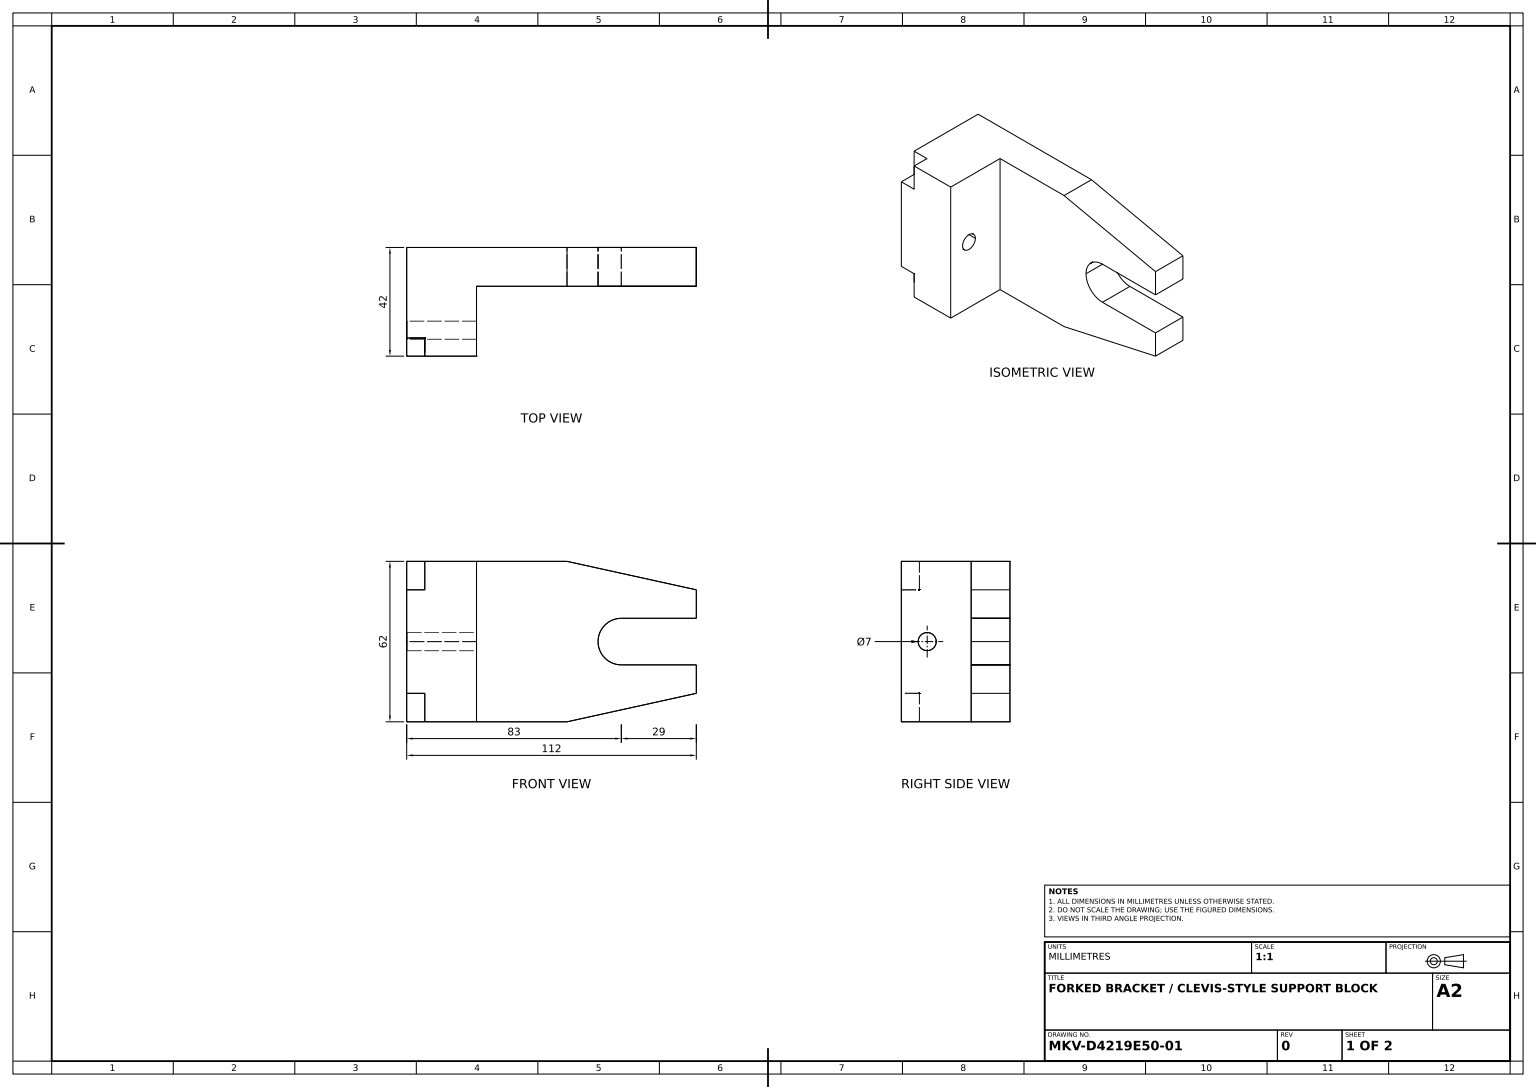
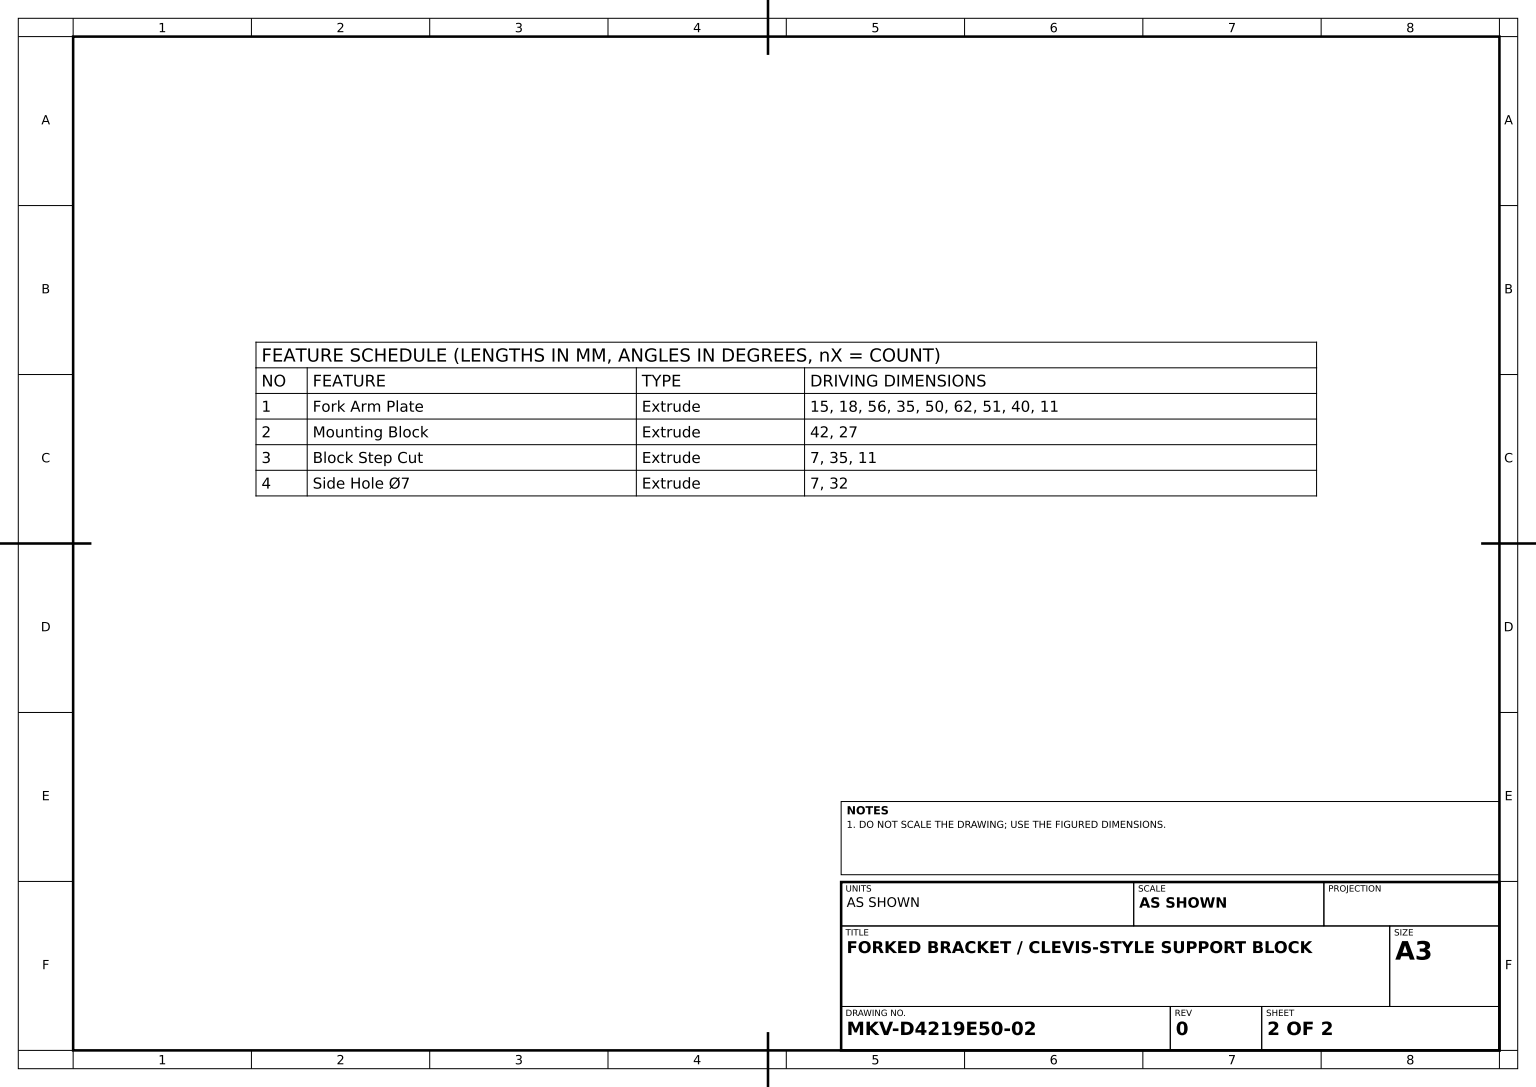
SolidWorks part; units mm, degrees
material "201 Annealed Stainless Steel (SS)"
ref_plane "Front Plane" through (0, 0, 0) normal (0, 0, 1) x (1, 0, 0)
ref_plane "Top Plane" through (0, 0, 0) normal (0, 1, 0) x (1, 0, 0)
ref_plane "Right Plane" through (0, 0, 0) normal (1, 0, 0) x (0, 0, -1)
sketch "Fork Arm Profile Sketch" plane through (0, 0, 0) normal (0, 0, 1) x (1, 0, 0)
  line L4 (85, 40) -> (85, 51)
  line L5 (0, 0) -> (0, 62)
  line L11 (0, 0) -> (35, 0)
  line L12 (0, 62) -> (35, 62)
  line L15 (85, 11) -> (85, 22)
  line L16 (56, 40) -> (85, 40)
  line L17 (56, 22) -> (85, 22)
  line L18 (85, 22) -> (85, 11)
  line L19 (35, 62) -> (85, 51)
  line L20 (35, 0) -> (85, 11)
  line L21 (85, 40) -> (85, 51)
  arc A1 (56, 40) -> (56, 22) centre (56, 31) ccw
  dimension "D1" = 18
  dimension "D3" = 35
  dimension "D2" = 56
  dimension "D4" = 50
  dimension "D5" = 62
  dimension "D6" = 51
  dimension "D7" = 40
  dimension "D8" = 11
  dimension "D9" = 35
extrude "Fork Arm Plate" add sketch "Fork Arm Profile Sketch" along normal blind 15 contours A1 L16 L4 L19 L12 L5 L11 L20 L15 L17
ref_plane "Plane1" through (0, 0, 0) normal (0, 0, 1) x (1, 0, 0)
sketch "Mounting Block Sketch" plane through (0, 0, 0) normal (0, 0, 1) x (1, 0, 0)
  line L0 (0, 62) -> (-27, 62)
  line L1 (-27, 62) -> (-27, 0)
  line L2 (-27, 0) -> (0, 0)
  line L3 (0, 62) -> (0, 0)
  dimension "D1" = 27
extrude "Mounting Block" add sketch "Mounting Block Sketch" along normal blind 42
sketch "Block Step Cut Sketch" plane through (-27, 0, 0) normal (-1, 0, 0) x (0, 0, 1)
  line L0 (42, 62) -> (42, 0)
  line L1 (42, 31) -> (42, 51)
  line L2 (42, 51) -> (35, 51)
  line L3 (35, 51) -> (35, 62)
  line L4 (42, 62) -> (0, 62) construction
  line L5 (35, 62) -> (42, 62)
  line L6 (42, 0) -> (35, 0)
  line L7 (42, 0) -> (0, 0) construction
  line L8 (35, 0) -> (35, 11)
  line L9 (35, 11) -> (42, 11)
  line L10 (0, 62) -> (0, 0) construction
  line M2 (0, 0) -> (42, 0)
  line M3 (42, 0) -> (42, 62)
  line M4 (42, 62) -> (0, 62)
  dimension "D1" = 35
  dimension "D2" = 11
extrude "Block Step Cut" cut sketch "Block Step Cut Sketch" against normal blind 7 contours L3 L2 M3 M4 | L9 L8 M2 M3
sketch "Side Hole Ø7 Sketch" plane through (-27, 0, 0) normal (-1, 0, 0) x (0, 0, 1)
  line L0 (42, 31) -> (32, 31) construction
  line L1 (42, 51) -> (42, 11) construction
  line L2 (0, 62) -> (0, 0) construction
  circle A0 centre (32, 31) radius 3.5
  dimension "D1" = 7
  dimension "D2" = 32
extrude "Side Hole Ø7" cut sketch "Side Hole Ø7 Sketch" against normal through all
